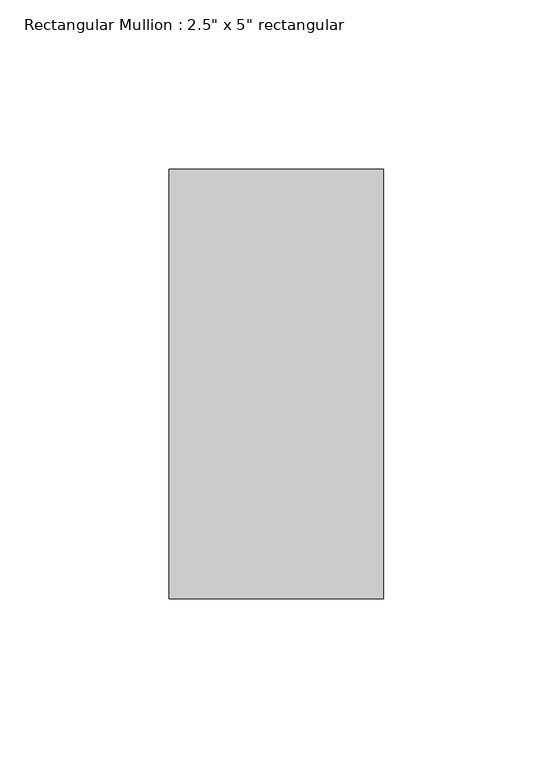
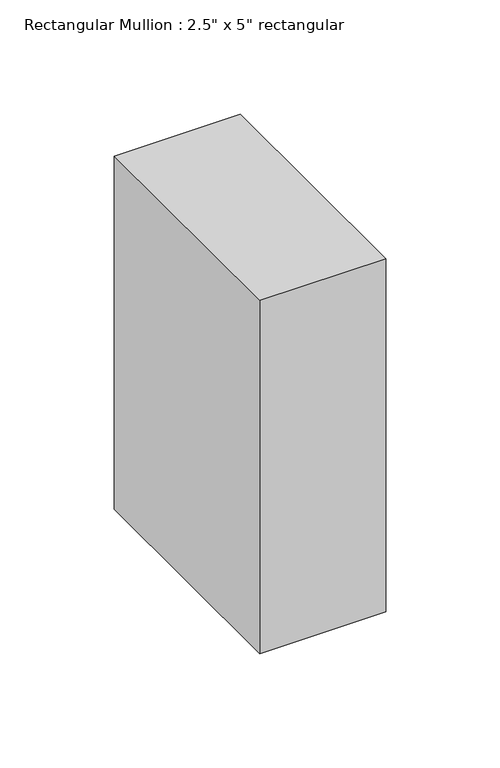
"""IFC4 building model written with IfcOpenShell, lengths in millimetres: member geometry."""

from ifc_helpers import new_model, si_unit, frame, origin, place, context, project, spatial, polyline, outline, extrude, source, transform, mapped, element, save


def member_95f02488(model_context):
    return source(origin(), model_context, "Body", "SweptSolid", [
        extrude(outline(polyline([(31.75, 63.5), (31.75, -63.5), (-31.75, -63.5), (-31.75, 63.5), (31.75, 63.5)])), frame((0.0, 0.0, -188.3833333), z_axis=(0.0, 0.0, 1.0), x_axis=(1.0, 0.0, 0.0)), (0.0, 0.0, 1.0), 188.3833333),
    ])


if __name__ == "__main__":
    model = new_model("IFC4")
    model_context = context("Model", 3, world=origin())
    ifc_project = project(units=[si_unit("LENGTHUNIT", "METRE", prefix="MILLI")], contexts=[model_context])
    site = spatial("IfcSite", under=ifc_project)
    building = spatial("IfcBuilding", under=site)
    placement = place(None, origin())
    member_shape = member_95f02488(model_context)
    element("IfcMember", 1, ObjectType="Rectangular Mullion : 2.5\" x 5\" rectangular", at=placement, inside=building, context=model_context, shape_type="MappedRepresentation", body=[
        mapped(member_shape, transform((0.0, 0.0, 0.0), x_axis=(1.0, 0.0, 0.0), y_axis=(0.0, 1.0, 0.0), z_axis=(0.0, 0.0, 1.0))),
    ])
    save(model, "model.ifc")

# Revit data of these elements
# Type "Rectangular Mullion : 2.5\" x 5\" rectangular"
#   built-in parameter 1007304 = 0.416667 (stored number, unit not read)
#   built-in parameter 1007301 = 0.104167 (stored number, unit not read)
#   built-in parameter 1007300 = 0.104167 (stored number, unit not read)
# Element 1 (IfcMember, "Rectangular Mullion : 2.5\" x 5\" rectangular")
#   Materials on its faces: "Aluminum"
# Materials
#   "Aluminum": class "Metal", colour RGB 247 247 247, transparency 0, Description = "Aluminum 6061", Cost = 0
